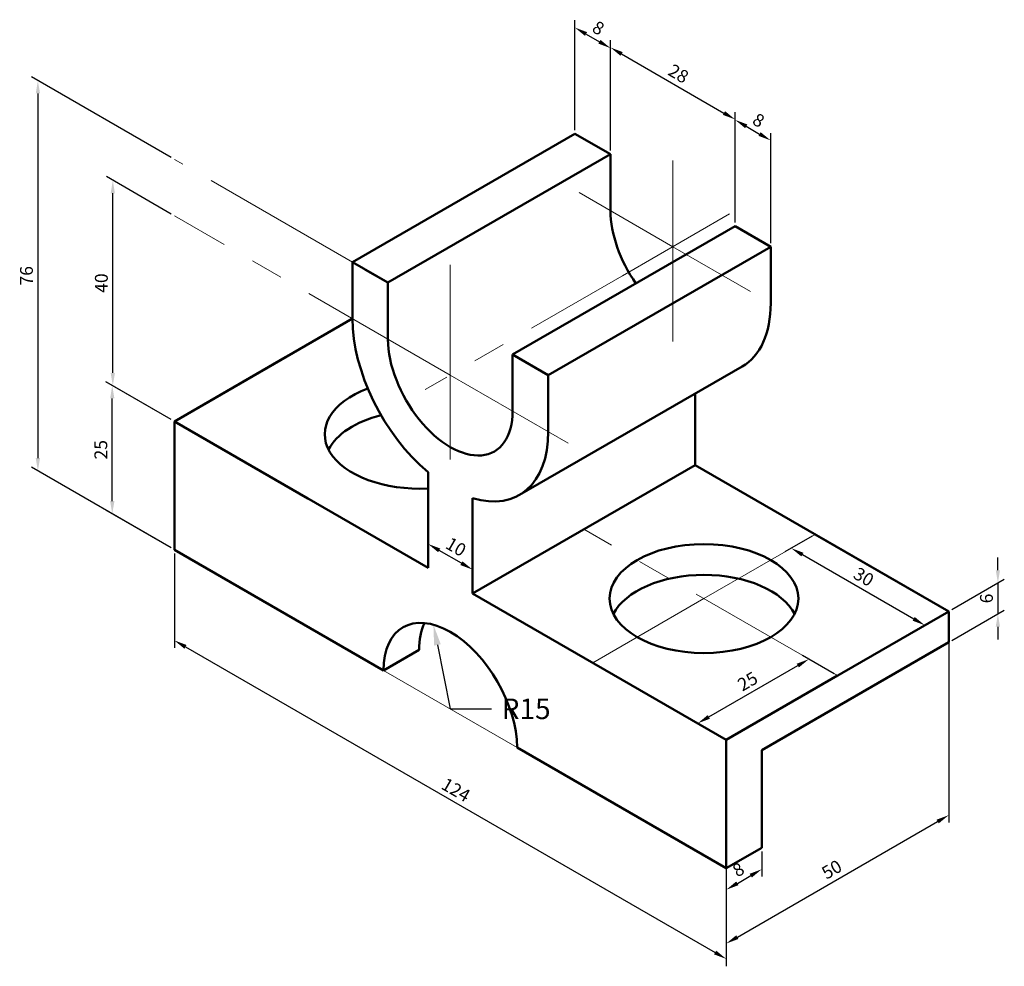
# Model space of a CAD drawing. Units: millimetres. Extents: x 595137 to 595329, y 444869 to 445053.
import ezdxf
from ezdxf import colors
from ezdxf.entities.mleader import LeaderData, LeaderLine
from ezdxf.math import Vec2, Vec3

# ---------------------------------------------------------------- set-up
doc = ezdxf.new("R2010")
doc.units = ezdxf.units.MM
doc.linetypes.add('CENTER', pattern=[50.8, 31.75, -6.35, 6.35, -6.35])
for name, color, linetype, lineweight in [('M-CNTR', 4, 'CENTER', 18), ('M-DIMS', 2, 'Continuous', 25), ('M-OUTL', 7, 'Continuous', 50)]:
    doc.layers.add(name, color=color, linetype=linetype, lineweight=lineweight)
doc.styles.get("Standard").update_dxf_attribs({"font": 'arial.ttf'})
doc.dimstyles.new('ISO-25', dxfattribs={"dimtxt": 2.5, "dimasz": 2.5, "dimexe": 1.25, "dimexo": 0.625, "dimtad": 1, "dimtxsty": 'Standard', "dimcen": 2.5, "dimadec": 0, "dimazin": 0, "dimtfac": 1, "dimtmove": 0, "dimatfit": 3, "dimfxl": 1, "dimarcsym": 0})

# ---------------------------------------------------------------- blocks, each defined once
blk = doc.blocks.new('*D1')
at = {"layer": 'Defpoints', "color": 0, "transparency": 16777216}
for p in [(595317.98, 444937.97), (595274.67, 444912.97), (595317.98, 444898.31)]:
    blk.add_point(p, dxfattribs=at)
at = {"layer": 'M-DIMS', "color": 0, "lineweight": -2, "transparency": 16777216}
for p, q in [((595317.98, 444937.25), (595317.98, 444896.87)), ((595274.67, 444912.25), (595274.67, 444871.87)), ((595276.84, 444874.56), (595315.81, 444897.06))]:
    blk.add_line(p, q, dxfattribs=at)
at = {"layer": 'M-DIMS', "color": 0, "transparency": 16777216}
for points in [[(595315.6, 444897.42), (595316.02, 444896.7), (595317.98, 444898.31)], [(595276.63, 444874.92), (595277.05, 444874.2), (595274.67, 444873.31)]]:
    blk.add_solid(points, dxfattribs=at)
at = {"layer": 'M-DIMS', "color": 0, "transparency": 16777216, "insert": (595295.37, 444887.46), "char_height": 2.5, "attachment_point": 5, "rotation": 30}
blk.add_mtext('50', dxfattribs=at)
blk = doc.blocks.new('*D2')
at = {"layer": 'Defpoints', "color": 0, "transparency": 16777216}
for p in [(595167.29, 444949.97), (595274.67, 444887.97), (595274.67, 444870.32)]:
    blk.add_point(p, dxfattribs=at)
at = {"layer": 'M-DIMS', "color": 0, "lineweight": -2, "transparency": 16777216}
for p, q in [((595167.29, 444949.25), (595167.29, 444930.88)), ((595169.45, 444931.07), (595272.51, 444871.57)), ((595274.67, 444887.25), (595274.67, 444868.88))]:
    blk.add_line(p, q, dxfattribs=at)
at = {"layer": 'M-DIMS', "color": 0, "transparency": 16777216}
for points in [[(595169.66, 444931.43), (595169.24, 444930.71), (595167.29, 444932.32)], [(595272.72, 444871.93), (595272.3, 444871.21), (595274.67, 444870.32)]]:
    blk.add_solid(points, dxfattribs=at)
at = {"layer": 'M-DIMS', "color": 0, "transparency": 16777216, "insert": (595221.92, 444902.95), "char_height": 2.5, "attachment_point": 5, "rotation": 330}
blk.add_mtext('124', dxfattribs=at)
blk = doc.blocks.new('*D3')
at = {"layer": 'Defpoints', "color": 0, "transparency": 16777216}
for p in [(595281.6, 444891.97), (595274.67, 444887.97), (595281.6, 444887.78)]:
    blk.add_point(p, dxfattribs=at)
at = {"layer": 'M-DIMS', "color": 0, "lineweight": -2, "transparency": 16777216}
for p, q in [((595281.6, 444891.25), (595281.6, 444886.34)), ((595274.67, 444887.25), (595274.67, 444882.34)), ((595276.84, 444885.03), (595279.44, 444886.53))]:
    blk.add_line(p, q, dxfattribs=at)
at = {"layer": 'M-DIMS', "color": 0, "transparency": 16777216}
for points in [[(595279.23, 444886.89), (595279.65, 444886.17), (595281.6, 444887.78)], [(595276.63, 444885.39), (595277.05, 444884.67), (595274.67, 444883.78)]]:
    blk.add_solid(points, dxfattribs=at)
at = {"layer": 'M-DIMS', "color": 0, "transparency": 16777216, "insert": (595277.19, 444887.43), "char_height": 2.5, "attachment_point": 5, "rotation": 30}
blk.add_mtext('8', dxfattribs=at)
blk = doc.blocks.new('*D4')
at = {"layer": 'Defpoints', "color": 0, "transparency": 16777216}
for p in [(595317.98, 444937.97), (595327.54, 444937.49), (595317.98, 444931.97)]:
    blk.add_point(p, dxfattribs=at)
at = {"layer": 'M-DIMS', "color": 0, "lineweight": -2, "transparency": 16777216}
for p, q in [((595327.54, 444945.99), (595327.54, 444948.49)), ((595318.6, 444938.33), (595328.79, 444944.22)), ((595327.54, 444943.49), (595327.54, 444937.49)), ((595318.6, 444932.33), (595328.79, 444938.22)), ((595327.54, 444934.99), (595327.54, 444932.49))]:
    blk.add_line(p, q, dxfattribs=at)
at = {"layer": 'M-DIMS', "color": 0, "transparency": 16777216}
for points in [[(595327.12, 444945.99), (595327.95, 444945.99), (595327.54, 444943.49)], [(595327.12, 444934.99), (595327.95, 444934.99), (595327.54, 444937.49)]]:
    blk.add_solid(points, dxfattribs=at)
at = {"layer": 'M-DIMS', "color": 0, "transparency": 16777216, "insert": (595325.64, 444940.49), "char_height": 2.5, "attachment_point": 5, "rotation": 90}
blk.add_mtext('6', dxfattribs=at)
blk = doc.blocks.new('*D5')
at = {"layer": 'Defpoints', "color": 0, "transparency": 16777216}
for p in [(595155.2, 444981.95), (595167.29, 444974.97), (595167.29, 444949.97)]:
    blk.add_point(p, dxfattribs=at)
at = {"layer": 'M-DIMS', "color": 0, "lineweight": -2, "transparency": 16777216}
for p, q in [((595166.66, 444975.33), (595153.95, 444982.67)), ((595155.2, 444959.45), (595155.2, 444979.45)), ((595166.66, 444950.33), (595153.95, 444957.67))]:
    blk.add_line(p, q, dxfattribs=at)
at = {"layer": 'M-DIMS', "color": 0, "transparency": 16777216}
for points in [[(595154.79, 444979.45), (595155.62, 444979.45), (595155.2, 444981.95)], [(595154.79, 444959.45), (595155.62, 444959.45), (595155.2, 444956.95)]]:
    blk.add_solid(points, dxfattribs=at)
at = {"layer": 'M-DIMS', "color": 0, "transparency": 16777216, "insert": (595153.3, 444969.45), "char_height": 2.5, "attachment_point": 5, "rotation": 90}
blk.add_mtext('25', dxfattribs=at)
blk = doc.blocks.new('*D6')
at = {"layer": 'Defpoints', "color": 0, "transparency": 16777216}
for p in [(595155.31, 445021.89), (595167.29, 445014.97), (595167.29, 444974.97)]:
    blk.add_point(p, dxfattribs=at)
at = {"layer": 'M-DIMS', "color": 0, "lineweight": -2, "transparency": 16777216}
for p, q in [((595166.66, 445015.33), (595154.06, 445022.61)), ((595155.31, 444984.39), (595155.31, 445019.39)), ((595166.66, 444975.33), (595154.06, 444982.61))]:
    blk.add_line(p, q, dxfattribs=at)
at = {"layer": 'M-DIMS', "color": 0, "transparency": 16777216}
for points in [[(595154.89, 445019.39), (595155.72, 445019.39), (595155.31, 445021.89)], [(595154.89, 444984.39), (595155.72, 444984.39), (595155.31, 444981.89)]]:
    blk.add_solid(points, dxfattribs=at)
at = {"layer": 'M-DIMS', "color": 0, "transparency": 16777216, "insert": (595153.4, 445001.89), "char_height": 2.5, "attachment_point": 5, "rotation": 90}
blk.add_mtext('40', dxfattribs=at)
blk = doc.blocks.new('*D7')
at = {"layer": 'Defpoints', "color": 0, "transparency": 16777216}
for p in [(595167.29, 445025.97), (595140.73, 444965.31), (595167.29, 444949.97)]:
    blk.add_point(p, dxfattribs=at)
at = {"layer": 'M-DIMS', "color": 0, "lineweight": -2, "transparency": 16777216}
for p, q in [((595166.66, 445026.33), (595139.48, 445042.03)), ((595140.73, 445038.81), (595140.73, 444967.81)), ((595166.66, 444950.33), (595139.48, 444966.03))]:
    blk.add_line(p, q, dxfattribs=at)
at = {"layer": 'M-DIMS', "color": 0, "transparency": 16777216}
for points in [[(595140.31, 445038.81), (595141.15, 445038.81), (595140.73, 445041.31)], [(595140.31, 444967.81), (595141.15, 444967.81), (595140.73, 444965.31)]]:
    blk.add_solid(points, dxfattribs=at)
at = {"layer": 'M-DIMS', "color": 0, "transparency": 16777216, "insert": (595138.83, 445003.31), "char_height": 2.5, "attachment_point": 5, "rotation": 90}
blk.add_mtext('76', dxfattribs=at)
blk = doc.blocks.new('*D8')
at = {"layer": 'Defpoints', "color": 0, "transparency": 16777216}
for p in [(595276.41, 445033.75), (595252.16, 445026.97), (595276.41, 445012.97)]:
    blk.add_point(p, dxfattribs=at)
at = {"layer": 'M-DIMS', "color": 0, "lineweight": -2, "transparency": 16777216}
for p, q in [((595252.16, 445027.69), (595252.16, 445049.19)), ((595254.32, 445046.5), (595274.24, 445035)), ((595276.41, 445013.69), (595276.41, 445035.19))]:
    blk.add_line(p, q, dxfattribs=at)
at = {"layer": 'M-DIMS', "color": 0, "transparency": 16777216}
for points in [[(595254.53, 445046.86), (595254.11, 445046.14), (595252.16, 445047.75)], [(595274.45, 445035.36), (595274.03, 445034.64), (595276.41, 445033.75)]]:
    blk.add_solid(points, dxfattribs=at)
at = {"layer": 'M-DIMS', "color": 0, "transparency": 16777216, "insert": (595265.23, 445042.39), "char_height": 2.5, "attachment_point": 5, "rotation": 330}
blk.add_mtext('28', dxfattribs=at)
blk = doc.blocks.new('*D9')
at = {"layer": 'Defpoints', "color": 0, "transparency": 16777216}
for p in [(595283.33, 445029.66), (595276.41, 445012.97), (595283.33, 445008.97)]:
    blk.add_point(p, dxfattribs=at)
at = {"layer": 'M-DIMS', "color": 0, "lineweight": -2, "transparency": 16777216}
for p, q in [((595276.41, 445013.69), (595276.41, 445035.1)), ((595278.57, 445032.41), (595281.17, 445030.91)), ((595283.33, 445009.69), (595283.33, 445031.1))]:
    blk.add_line(p, q, dxfattribs=at)
at = {"layer": 'M-DIMS', "color": 0, "transparency": 16777216}
for points in [[(595278.78, 445032.77), (595278.36, 445032.05), (595276.41, 445033.66)], [(595281.38, 445031.27), (595280.96, 445030.55), (595283.33, 445029.66)]]:
    blk.add_solid(points, dxfattribs=at)
at = {"layer": 'M-DIMS', "color": 0, "transparency": 16777216, "insert": (595280.82, 445033.31), "char_height": 2.5, "attachment_point": 5, "rotation": 330}
blk.add_mtext('8', dxfattribs=at)
blk = doc.blocks.new('*D10')
at = {"layer": 'Defpoints', "color": 0, "transparency": 16777216}
for p in [(595252.16, 445047.63), (595245.23, 445030.97), (595252.16, 445026.97)]:
    blk.add_point(p, dxfattribs=at)
at = {"layer": 'M-DIMS', "color": 0, "lineweight": -2, "transparency": 16777216}
for p, q in [((595245.23, 445031.69), (595245.23, 445053.07)), ((595247.39, 445050.38), (595249.99, 445048.88)), ((595252.16, 445027.69), (595252.16, 445049.07))]:
    blk.add_line(p, q, dxfattribs=at)
at = {"layer": 'M-DIMS', "color": 0, "transparency": 16777216}
for points in [[(595247.6, 445050.74), (595247.19, 445050.02), (595245.23, 445051.63)], [(595250.2, 445049.24), (595249.78, 445048.52), (595252.16, 445047.63)]]:
    blk.add_solid(points, dxfattribs=at)
at = {"layer": 'M-DIMS', "color": 0, "transparency": 16777216, "insert": (595249.64, 445051.28), "char_height": 2.5, "attachment_point": 5, "rotation": 330}
blk.add_mtext('8', dxfattribs=at)
blk = doc.blocks.new('*D11')
at = {"layer": 'Defpoints', "color": 0, "transparency": 16777216}
for p in [(595290.77, 444928.68), (595296.32, 444925.47), (595274.67, 444912.97)]:
    blk.add_point(p, dxfattribs=at)
at = {"layer": 'M-DIMS', "color": 0, "lineweight": -2, "transparency": 16777216}
for p, q in [((595295.7, 444925.83), (595289.52, 444929.4)), ((595271.29, 444917.43), (595288.61, 444927.43)), ((595274.05, 444913.33), (595267.87, 444916.9))]:
    blk.add_line(p, q, dxfattribs=at)
at = {"layer": 'M-DIMS', "color": 0, "transparency": 16777216}
for points in [[(595288.4, 444927.79), (595288.81, 444927.07), (595290.77, 444928.68)], [(595271.08, 444917.79), (595271.49, 444917.07), (595269.12, 444916.18)]]:
    blk.add_solid(points, dxfattribs=at)
at = {"layer": 'M-DIMS', "color": 0, "transparency": 16777216, "insert": (595279, 444924.08), "char_height": 2.5, "attachment_point": 5, "rotation": 30}
blk.add_mtext('25', dxfattribs=at)
blk = doc.blocks.new('*D12')
at = {"layer": 'Defpoints', "color": 0, "transparency": 16777216}
for p in [(595291.99, 444952.97), (595317.98, 444937.97), (595313.31, 444935.28)]:
    blk.add_point(p, dxfattribs=at)
at = {"layer": 'M-DIMS', "color": 0, "lineweight": -2, "transparency": 16777216}
for p, q in [((595291.37, 444952.61), (595286.08, 444949.56)), ((595289.5, 444949.03), (595311.15, 444936.53)), ((595317.35, 444937.61), (595312.06, 444934.56))]:
    blk.add_line(p, q, dxfattribs=at)
at = {"layer": 'M-DIMS', "color": 0, "transparency": 16777216}
for points in [[(595289.7, 444949.39), (595289.29, 444948.67), (595287.33, 444950.28)], [(595311.36, 444936.89), (595310.94, 444936.17), (595313.31, 444935.28)]]:
    blk.add_solid(points, dxfattribs=at)
at = {"layer": 'M-DIMS', "color": 0, "transparency": 16777216, "insert": (595301.27, 444944.43), "char_height": 2.5, "attachment_point": 5, "rotation": 330}
blk.add_mtext('30', dxfattribs=at)
blk = doc.blocks.new('*D13')
at = {"layer": 'Defpoints', "color": 0, "transparency": 16777216}
for p in [(595216.65, 444951.11), (595216.65, 444946.47), (595225.31, 444941.47)]:
    blk.add_point(p, dxfattribs=at)
at = {"layer": 'M-DIMS', "color": 0, "lineweight": -2, "transparency": 16777216}
for p, q in [((595216.65, 444947.19), (595216.65, 444952.56)), ((595223.15, 444947.36), (595218.82, 444949.86)), ((595225.31, 444942.19), (595225.31, 444947.56))]:
    blk.add_line(p, q, dxfattribs=at)
at = {"layer": 'M-DIMS', "color": 0, "transparency": 16777216}
for points in [[(595219.02, 444950.22), (595218.61, 444949.5), (595216.65, 444951.11)], [(595223.35, 444947.72), (595222.94, 444947), (595225.31, 444946.11)]]:
    blk.add_solid(points, dxfattribs=at)
at = {"layer": 'M-DIMS', "color": 0, "transparency": 16777216, "insert": (595221.93, 444950.26), "char_height": 2.5, "attachment_point": 5, "rotation": 330}
blk.add_mtext('10', dxfattribs=at)

msp = doc.modelspace()

# ---------------------------------------------------------------- linework, layer by layer
at = {"layer": 'M-CNTR'}
for p, q in [((595201.928, 445005.973), (595167.287, 445025.973)), ((595264.281, 445008.973), (595264.281, 445025.754)), ((595264.281, 445008.973), (595246.048, 445019.5)), ((595220.98, 444983.973), (595167.287, 445014.973)), ((595254.474, 445003.31), (595275.32, 445015.346)), ((595264.281, 445008.973), (595216.086, 444981.147)), ((595264.281, 445008.973), (595279.41, 445000.239)), ((595264.281, 445008.973), (595264.281, 444990.528)), ((595220.98, 444983.973), (595220.98, 445005.45)), ((595220.98, 444983.973), (595220.98, 444967.549)), ((595220.98, 444983.973), (595243.906, 444970.737)), ((595296.324, 444925.473), (595246.961, 444953.973)), ((595270.344, 444940.473), (595291.994, 444952.973)), ((595270.344, 444940.473), (595248.693, 444927.973)), ((595207.99, 444926.473), (595233.971, 444911.473))]:
    msp.add_line(p, q, dxfattribs=at)
at = {"layer": 'M-OUTL'}
for p, q in [((595201.928, 445005.973), (595245.229, 445030.973)), ((595245.229, 445030.973), (595252.157, 445026.973)), ((595208.856, 445001.973), (595252.157, 445026.973)), ((595252.157, 445015.973), (595252.157, 445026.973)), ((595233.105, 444987.973), (595276.406, 445012.973)), ((595276.406, 445012.973), (595283.334, 445008.973)), ((595240.033, 444983.973), (595283.334, 445008.973)), ((595283.334, 444997.973), (595283.334, 445008.973)), ((595201.928, 445005.973), (595208.856, 445001.973)), ((595201.928, 444994.973), (595201.928, 445005.973)), ((595208.856, 445001.973), (595204.48, 445004.499)), ((595208.856, 444990.973), (595208.856, 445001.973)), ((595167.287, 444974.973), (595201.928, 444994.973)), ((595167.287, 444974.973), (595188.937, 444987.473)), ((595233.105, 444976.973), (595233.105, 444987.973)), ((595233.105, 444987.973), (595240.033, 444983.973)), ((595234.452, 444960.638), (595277.754, 444985.638)), ((595240.033, 444972.973), (595240.033, 444983.973)), ((595268.612, 444966.473), (595268.612, 444980.36)), ((595167.287, 444974.973), (595167.287, 444949.973)), ((595167.287, 444974.973), (595193.267, 444959.973)), ((595167.287, 444949.973), (595167.287, 444974.973)), ((595167.287, 444949.973), (595167.287, 444974.973)), ((595216.65, 444946.473), (595167.287, 444974.973)), ((595225.31, 444941.473), (595268.612, 444966.473)), ((595268.612, 444966.473), (595317.975, 444937.973)), ((595216.65, 444946.473), (595216.65, 444965.049)), ((595225.31, 444941.473), (595225.31, 444960.049)), ((595317.975, 444937.973), (595291.994, 444952.973)), ((595167.287, 444949.973), (595207.99, 444926.473)), ((595274.674, 444912.973), (595225.31, 444941.473)), ((595317.975, 444937.973), (595274.674, 444912.973)), ((595317.975, 444937.973), (595317.975, 444931.973)), ((595317.975, 444931.973), (595281.602, 444910.973)), ((595207.99, 444926.473), (595214.918, 444930.473)), ((595274.674, 444912.973), (595296.324, 444925.473)), ((595274.674, 444887.973), (595274.674, 444912.973)), ((595233.971, 444911.473), (595274.674, 444887.973)), ((595281.602, 444891.973), (595281.602, 444910.973)), ((595274.674, 444887.973), (595281.602, 444891.973))]:
    msp.add_line(p, q, dxfattribs=at)
for centre, major_axis, start_param, end_param in [((595264.281, 445008.973), (8.573, -14.849), 3.9269908, 4.8644977), ((595264.281, 445008.973), (13.472, -23.335), 6.2831853, 7.0685835), ((595220.98, 444983.973), (13.472, -23.335), 3.9269908, 5.2685109), ((595220.98, 444983.973), (8.573, -14.849), 3.9269908, 7.0685835), ((595214.918, 444972.473), (-18.371, 0), 5.2869595, 7.9484028), ((595214.918, 444966.473), (-18.371, 0), 5.1270758, 5.9964288), ((595220.98, 444983.973), (13.472, -23.335), 5.7270633, 7.0685835), ((595270.344, 444934.473), (-18.371, 0), 3.4283492, 5.9964288), ((595220.98, 444918.973), (9.186, -15.91), 0.7853982, 3.9269908), ((595227.908, 444922.973), (9.186, -15.91), 3.5282813, 3.9269908)]:
    msp.add_ellipse(centre, major_axis=major_axis, ratio=0.5773503, start_param=start_param, end_param=end_param, dxfattribs=at)
msp.add_ellipse((595270.344, 444940.473), major_axis=(-18.371, 0), ratio=0.5773503, dxfattribs=at)

# ---------------------------------------------------------------- dimensions: what is measured, and where the dimension line sits
at = {"layer": 'M-DIMS'}
for p1, p2, distance, picture, middle in [((595245.229, 445030.973), (595252.157, 445026.973), 17.89, '*D10', (595249.644, 445051.277)), ((595252.157, 445026.973), (595276.406, 445012.973), 17.991, '*D8', (595265.232, 445042.394)), ((595167.287, 445025.973), (595167.287, 444949.973), -26.557, '*D7', (595138.829, 445003.305)), ((595276.406, 445012.973), (595283.334, 445008.973), 17.917, '*D9', (595280.821, 445033.308)), ((595167.287, 444974.973), (595167.287, 445014.973), 11.981, '*D6', (595153.404, 445001.89)), ((595167.287, 444949.973), (595167.287, 444974.973), 12.083, '*D5', (595153.302, 444969.449)), ((595225.31, 444941.473), (595216.65, 444946.473), -4.017, '*D13', (595221.931, 444950.258)), ((595291.994, 444952.973), (595317.975, 444937.973), -4.663, '*D12', (595301.273, 444944.428)), ((595167.287, 444949.973), (595274.674, 444887.973), -15.288, '*D2', (595221.92, 444902.948)), ((595317.975, 444937.973), (595317.975, 444931.973), 9.563, '*D4', (595325.636, 444940.494)), ((595274.674, 444912.973), (595317.975, 444937.973), -34.348, '*D1', (595295.374, 444887.458)), ((595274.674, 444912.973), (595296.324, 444925.473), 5.553, '*D11', (595278.995, 444924.076)), ((595274.674, 444887.973), (595281.602, 444891.973), -3.632, '*D3', (595277.187, 444887.426))]:
    dim = msp.add_aligned_dim(p1=p1, p2=p2, distance=distance, dimstyle='ISO-25', override={"dimclrd": 0, "dimclre": 0, "dimclrt": 0}, dxfattribs=at)
    dim.commit()
    dim.dimension.update_dxf_attribs({"geometry": picture, "text_midpoint": middle})

# ---------------------------------------------------------------- leaders
ml = msp.add_multileader_mtext('Standard', dxfattribs=at)
ml.set_content('R15', color=256)
ml.set_leader_properties()
ml.build(insert=Vec2(0, 0))
ctx = ml.context
ctx.base_point, ctx.plane_origin = Vec3(595228.98, 444918.973), Vec3(595217.691, 444935.383)
notes = []
notes.append((ctx, [(0, (1, 1, 0), (595220.98, 444918.973), (1, 0), 8, [(0, [(595217.691, 444935.383)], 0, [])])]))
ctx.mtext.insert, ctx.mtext.flow_direction = Vec3(595230.98, 444921.007), 5
for ctx, leaders in notes:
    for number, flags, end, landing, length, lines in leaders:
        leader = LeaderData()
        leader.index, (leader.has_last_leader_line, leader.has_dogleg_vector, leader.attachment_direction) = number, flags
        leader.last_leader_point, leader.dogleg_vector, leader.dogleg_length = Vec3(end), Vec3(landing), length
        for number, points, colour, breaks in lines:
            line = LeaderLine()
            line.index, line.vertices, line.color, line.breaks = number, Vec3.list(points), colors.encode_raw_color(colour), breaks
            leader.lines.append(line)
        ctx.leaders.append(leader)

doc.saveas('drawing.dxf')
